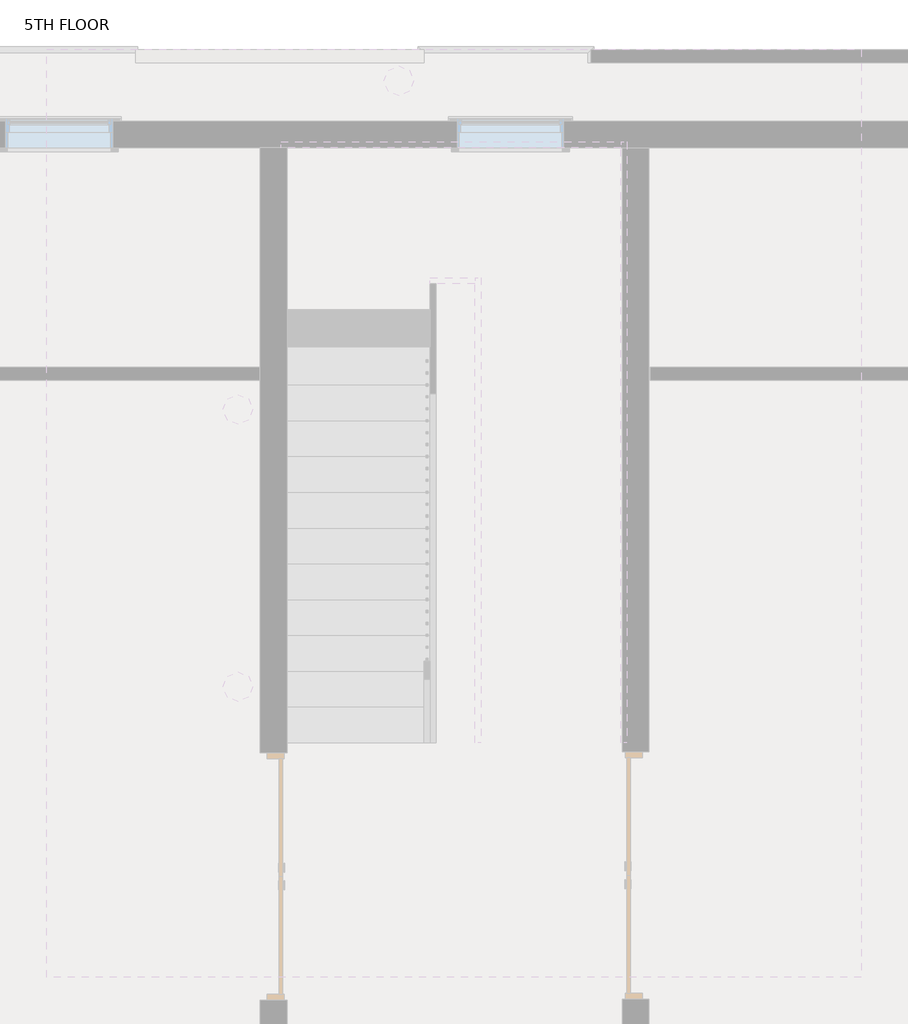
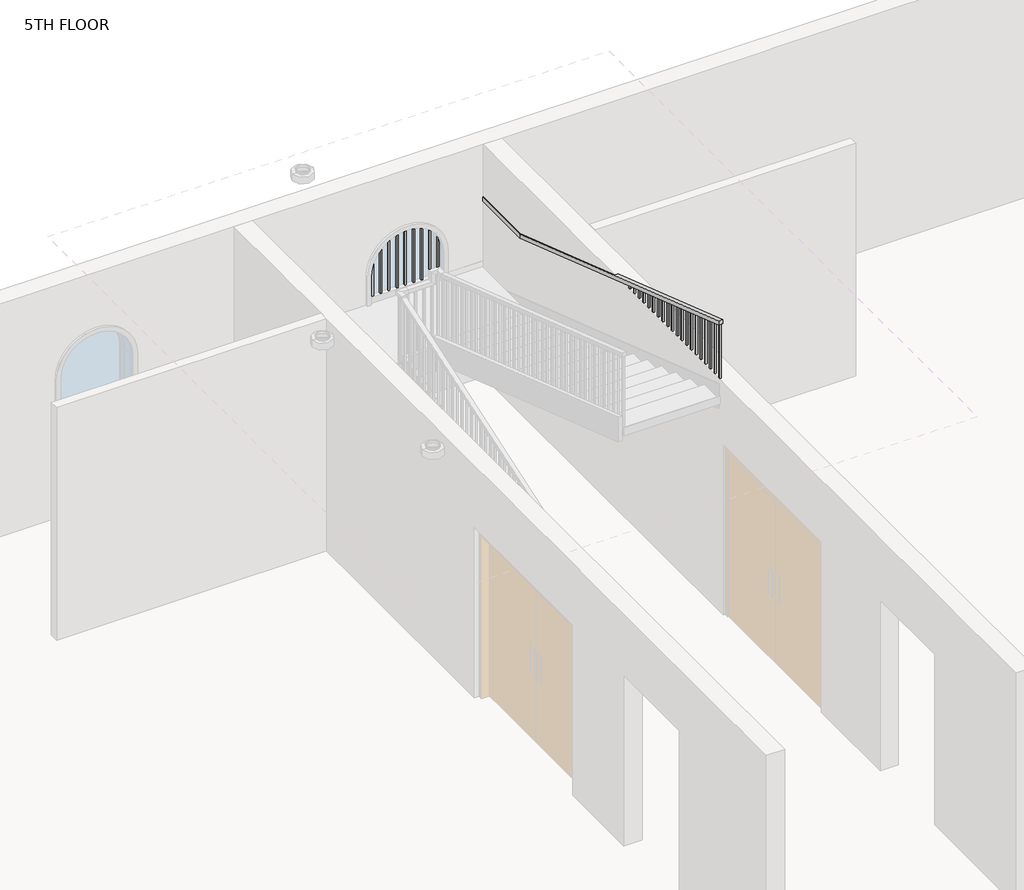
# One storey, part 5 of 7: 1 railing.
"""IFC4 building model written with IfcOpenShell, lengths in millimetres."""

from ifc_helpers import new_model, si_unit, frame, origin, place, context, project, spatial, polyline, outline, extrude, faceted_brep, element, save

model = new_model("IFC4")

# Units and contexts
model_context = context("Model", 3, world=origin())
ifc_project = project(units=[si_unit("LENGTHUNIT", "METRE", prefix="MILLI")], contexts=[model_context])

# Site, building, storey
site = spatial("IfcSite", under=ifc_project)
building = spatial("IfcBuilding", under=site)
storey = spatial("IfcBuildingStorey", under=building, Name="5TH FLOOR", Elevation=16002.0)

# Railing
placement = place(None, origin())
element("IfcRailing", 1, ObjectType="Handrail - Rectangular", at=placement, inside=storey, context=model_context, shape_type="SolidModel", body=[
    faceted_brep([(-1899.5987998, 2564.5067329, 17019.8142857), (-1899.5987998, 2564.5067329, 16966.1699957), (-1848.7987998, 2564.5067329, 16966.1699957), (-1848.7987998, 2564.5067329, 17019.8142857), (-1899.5987998, 6526.9067329, 18364.2), (-1899.5987998, 6535.2899033, 18313.4), (-1848.7987998, 6535.2899033, 18313.4), (-1848.7987998, 6526.9067329, 18364.2), (-1899.5987998, 7682.6067329, 18313.4), (-1899.5987998, 7682.6067329, 18364.2), (1046.8012002, 7682.6067329, 18364.2), (1046.8012002, 7682.6067329, 18313.4), (-1848.7987998, 7631.8067329, 18313.4), (996.0012002, 7631.8067329, 18313.4), (-1848.7987998, 7631.8067329, 18364.2), (996.0012002, 7631.8067329, 18364.2), (1046.8012002, 6831.7067329, 18364.2), (1046.8012002, 6823.3235624, 18313.4), (996.0012002, 6823.3235624, 18313.4), (996.0012002, 6831.7067329, 18364.2), (1046.8012002, 2564.5067329, 19812.0), (996.0012002, 2564.5067329, 19812.0), (996.0012002, 2564.5067329, 19758.35571), (1046.8012002, 2564.5067329, 19758.35571)], [[[0, 1, 2, 3]], [[1, 0, 4, 5]], [[2, 1, 5, 6]], [[3, 2, 6, 7]], [[0, 3, 7, 4]], [[8, 9, 10, 11]], [[12, 8, 11, 13]], [[14, 12, 13, 15]], [[9, 14, 15, 10]], [[11, 10, 16, 17]], [[13, 11, 17, 18]], [[15, 13, 18, 19]], [[10, 15, 19, 16]], [[5, 4, 9, 8]], [[6, 5, 8, 12]], [[7, 6, 12, 14]], [[4, 7, 14, 9]], [[20, 21, 22, 23]], [[17, 16, 20, 23]], [[18, 17, 23, 22]], [[19, 18, 22, 21]], [[16, 19, 21, 20]]]),
    extrude(outline(polyline([(2586.7317329, 19750.815085), (2586.7317329, 18979.8831452), (2567.6817329, 18986.3465381), (2567.6817329, 19757.2784779), (2586.7317329, 19750.815085)])), frame((1011.8762002, 0.0, 0.0), z_axis=(1.0, 0.0, 0.0), x_axis=(0.0, 1.0, 0.0)), (0.0, 0.0, 1.0), 19.05),
    extrude(outline(polyline([(2688.3317329, 19716.3436565), (2688.3317329, 18945.4117167), (2669.2817329, 18951.8751095), (2669.2817329, 19722.8070493), (2688.3317329, 19716.3436565)])), frame((1011.8762002, 0.0, 0.0), z_axis=(1.0, 0.0, 0.0), x_axis=(0.0, 1.0, 0.0)), (0.0, 0.0, 1.0), 19.05),
    extrude(outline(polyline([(2789.9317329, 19681.8722279), (2789.9317329, 18910.9402881), (2770.8817329, 18917.403681), (2770.8817329, 19688.3356207), (2789.9317329, 19681.8722279)])), frame((1011.8762002, 0.0, 0.0), z_axis=(1.0, 0.0, 0.0), x_axis=(0.0, 1.0, 0.0)), (0.0, 0.0, 1.0), 19.05),
    extrude(outline(polyline([(2891.5317329, 19647.4007993), (2891.5317329, 18876.4688595), (2872.4817329, 18882.9322524), (2872.4817329, 19653.8641922), (2891.5317329, 19647.4007993)])), frame((1011.8762002, 0.0, 0.0), z_axis=(1.0, 0.0, 0.0), x_axis=(0.0, 1.0, 0.0)), (0.0, 0.0, 1.0), 19.05),
    extrude(outline(polyline([(2993.1317329, 19612.9293707), (2993.1317329, 18841.997431), (2974.0817329, 18848.4608238), (2974.0817329, 19619.3927636), (2993.1317329, 19612.9293707)])), frame((1011.8762002, 0.0, 0.0), z_axis=(1.0, 0.0, 0.0), x_axis=(0.0, 1.0, 0.0)), (0.0, 0.0, 1.0), 19.05),
    extrude(outline(polyline([(3094.7317329, 19578.4579422), (3094.7317329, 18807.5260024), (3075.6817329, 18813.9893952), (3075.6817329, 19584.921335), (3094.7317329, 19578.4579422)])), frame((1011.8762002, 0.0, 0.0), z_axis=(1.0, 0.0, 0.0), x_axis=(0.0, 1.0, 0.0)), (0.0, 0.0, 1.0), 19.05),
    extrude(outline(polyline([(3196.3317329, 19543.9865136), (3196.3317329, 18773.0545738), (3177.2817329, 18779.5179667), (3177.2817329, 19550.4499065), (3196.3317329, 19543.9865136)])), frame((1011.8762002, 0.0, 0.0), z_axis=(1.0, 0.0, 0.0), x_axis=(0.0, 1.0, 0.0)), (0.0, 0.0, 1.0), 19.05),
    extrude(outline(polyline([(3297.9317329, 19509.515085), (3297.9317329, 18738.5831452), (3278.8817329, 18745.0465381), (3278.8817329, 19515.9784779), (3297.9317329, 19509.515085)])), frame((1011.8762002, 0.0, 0.0), z_axis=(1.0, 0.0, 0.0), x_axis=(0.0, 1.0, 0.0)), (0.0, 0.0, 1.0), 19.05),
    extrude(outline(polyline([(3399.5317329, 19475.0436565), (3399.5317329, 18704.1117167), (3380.4817329, 18710.5751095), (3380.4817329, 19481.5070493), (3399.5317329, 19475.0436565)])), frame((1011.8762002, 0.0, 0.0), z_axis=(1.0, 0.0, 0.0), x_axis=(0.0, 1.0, 0.0)), (0.0, 0.0, 1.0), 19.05),
    extrude(outline(polyline([(3501.1317329, 19440.5722279), (3501.1317329, 18669.6402881), (3482.0817329, 18676.103681), (3482.0817329, 19447.0356207), (3501.1317329, 19440.5722279)])), frame((1011.8762002, 0.0, 0.0), z_axis=(1.0, 0.0, 0.0), x_axis=(0.0, 1.0, 0.0)), (0.0, 0.0, 1.0), 19.05),
    extrude(outline(polyline([(3602.7317329, 19406.1007993), (3602.7317329, 18635.1688595), (3583.6817329, 18641.6322524), (3583.6817329, 19412.5641922), (3602.7317329, 19406.1007993)])), frame((1011.8762002, 0.0, 0.0), z_axis=(1.0, 0.0, 0.0), x_axis=(0.0, 1.0, 0.0)), (0.0, 0.0, 1.0), 19.05),
    extrude(outline(polyline([(3704.3317329, 19371.6293707), (3704.3317329, 18600.697431), (3685.2817329, 18607.1608238), (3685.2817329, 19378.0927636), (3704.3317329, 19371.6293707)])), frame((1011.8762002, 0.0, 0.0), z_axis=(1.0, 0.0, 0.0), x_axis=(0.0, 1.0, 0.0)), (0.0, 0.0, 1.0), 19.05),
    extrude(outline(polyline([(3805.9317329, 19337.1579422), (3805.9317329, 18566.2260024), (3786.8817329, 18572.6893952), (3786.8817329, 19343.621335), (3805.9317329, 19337.1579422)])), frame((1011.8762002, 0.0, 0.0), z_axis=(1.0, 0.0, 0.0), x_axis=(0.0, 1.0, 0.0)), (0.0, 0.0, 1.0), 19.05),
    extrude(outline(polyline([(3907.5317329, 19302.6865136), (3907.5317329, 18531.7545738), (3888.4817329, 18538.2179667), (3888.4817329, 19309.1499065), (3907.5317329, 19302.6865136)])), frame((1011.8762002, 0.0, 0.0), z_axis=(1.0, 0.0, 0.0), x_axis=(0.0, 1.0, 0.0)), (0.0, 0.0, 1.0), 19.05),
    extrude(outline(polyline([(4009.1317329, 19268.215085), (4009.1317329, 18497.2831452), (3990.0817329, 18503.7465381), (3990.0817329, 19274.6784779), (4009.1317329, 19268.215085)])), frame((1011.8762002, 0.0, 0.0), z_axis=(1.0, 0.0, 0.0), x_axis=(0.0, 1.0, 0.0)), (0.0, 0.0, 1.0), 19.05),
    extrude(outline(polyline([(4110.7317329, 19233.7436565), (4110.7317329, 18462.8117167), (4091.6817329, 18469.2751095), (4091.6817329, 19240.2070493), (4110.7317329, 19233.7436565)])), frame((1011.8762002, 0.0, 0.0), z_axis=(1.0, 0.0, 0.0), x_axis=(0.0, 1.0, 0.0)), (0.0, 0.0, 1.0), 19.05),
    extrude(outline(polyline([(4212.3317329, 19199.2722279), (4212.3317329, 18428.3402881), (4193.2817329, 18434.803681), (4193.2817329, 19205.7356207), (4212.3317329, 19199.2722279)])), frame((1011.8762002, 0.0, 0.0), z_axis=(1.0, 0.0, 0.0), x_axis=(0.0, 1.0, 0.0)), (0.0, 0.0, 1.0), 19.05),
    extrude(outline(polyline([(4313.9317329, 19164.8007993), (4313.9317329, 18393.8688595), (4294.8817329, 18400.3322524), (4294.8817329, 19171.2641922), (4313.9317329, 19164.8007993)])), frame((1011.8762002, 0.0, 0.0), z_axis=(1.0, 0.0, 0.0), x_axis=(0.0, 1.0, 0.0)), (0.0, 0.0, 1.0), 19.05),
    extrude(outline(polyline([(4415.5317329, 19130.3293707), (4415.5317329, 18359.397431), (4396.4817329, 18365.8608238), (4396.4817329, 19136.7927636), (4415.5317329, 19130.3293707)])), frame((1011.8762002, 0.0, 0.0), z_axis=(1.0, 0.0, 0.0), x_axis=(0.0, 1.0, 0.0)), (0.0, 0.0, 1.0), 19.05),
    extrude(outline(polyline([(4517.1317329, 19095.8579422), (4517.1317329, 18324.9260024), (4498.0817329, 18331.3893952), (4498.0817329, 19102.321335), (4517.1317329, 19095.8579422)])), frame((1011.8762002, 0.0, 0.0), z_axis=(1.0, 0.0, 0.0), x_axis=(0.0, 1.0, 0.0)), (0.0, 0.0, 1.0), 19.05),
    extrude(outline(polyline([(4618.7317329, 19061.3865136), (4618.7317329, 18290.4545738), (4599.6817329, 18296.9179667), (4599.6817329, 19067.8499065), (4618.7317329, 19061.3865136)])), frame((1011.8762002, 0.0, 0.0), z_axis=(1.0, 0.0, 0.0), x_axis=(0.0, 1.0, 0.0)), (0.0, 0.0, 1.0), 19.05),
    extrude(outline(polyline([(4720.3317329, 19026.915085), (4720.3317329, 18255.9831452), (4701.2817329, 18262.4465381), (4701.2817329, 19033.3784779), (4720.3317329, 19026.915085)])), frame((1011.8762002, 0.0, 0.0), z_axis=(1.0, 0.0, 0.0), x_axis=(0.0, 1.0, 0.0)), (0.0, 0.0, 1.0), 19.05),
    extrude(outline(polyline([(4821.9317329, 18992.4436565), (4821.9317329, 18221.5117167), (4802.8817329, 18227.9751095), (4802.8817329, 18998.9070493), (4821.9317329, 18992.4436565)])), frame((1011.8762002, 0.0, 0.0), z_axis=(1.0, 0.0, 0.0), x_axis=(0.0, 1.0, 0.0)), (0.0, 0.0, 1.0), 19.05),
    extrude(outline(polyline([(4923.5317329, 18957.9722279), (4923.5317329, 18187.0402881), (4904.4817329, 18193.503681), (4904.4817329, 18964.4356207), (4923.5317329, 18957.9722279)])), frame((1011.8762002, 0.0, 0.0), z_axis=(1.0, 0.0, 0.0), x_axis=(0.0, 1.0, 0.0)), (0.0, 0.0, 1.0), 19.05),
    extrude(outline(polyline([(5025.1317329, 18923.5007993), (5025.1317329, 18152.5688595), (5006.0817329, 18159.0322524), (5006.0817329, 18929.9641922), (5025.1317329, 18923.5007993)])), frame((1011.8762002, 0.0, 0.0), z_axis=(1.0, 0.0, 0.0), x_axis=(0.0, 1.0, 0.0)), (0.0, 0.0, 1.0), 19.05),
    extrude(outline(polyline([(5126.7317329, 18889.0293707), (5126.7317329, 18118.097431), (5107.6817329, 18124.5608238), (5107.6817329, 18895.4927636), (5126.7317329, 18889.0293707)])), frame((1011.8762002, 0.0, 0.0), z_axis=(1.0, 0.0, 0.0), x_axis=(0.0, 1.0, 0.0)), (0.0, 0.0, 1.0), 19.05),
    extrude(outline(polyline([(5228.3317329, 18854.5579422), (5228.3317329, 18083.6260024), (5209.2817329, 18090.0893952), (5209.2817329, 18861.021335), (5228.3317329, 18854.5579422)])), frame((1011.8762002, 0.0, 0.0), z_axis=(1.0, 0.0, 0.0), x_axis=(0.0, 1.0, 0.0)), (0.0, 0.0, 1.0), 19.05),
    extrude(outline(polyline([(5329.9317329, 18820.0865136), (5329.9317329, 18049.1545738), (5310.8817329, 18055.6179667), (5310.8817329, 18826.5499065), (5329.9317329, 18820.0865136)])), frame((1011.8762002, 0.0, 0.0), z_axis=(1.0, 0.0, 0.0), x_axis=(0.0, 1.0, 0.0)), (0.0, 0.0, 1.0), 19.05),
    extrude(outline(polyline([(5431.5317329, 18785.615085), (5431.5317329, 18014.6831452), (5412.4817329, 18021.1465381), (5412.4817329, 18792.0784779), (5431.5317329, 18785.615085)])), frame((1011.8762002, 0.0, 0.0), z_axis=(1.0, 0.0, 0.0), x_axis=(0.0, 1.0, 0.0)), (0.0, 0.0, 1.0), 19.05),
    extrude(outline(polyline([(5533.1317329, 18751.1436565), (5533.1317329, 17980.2117167), (5514.0817329, 17986.6751095), (5514.0817329, 18757.6070493), (5533.1317329, 18751.1436565)])), frame((1011.8762002, 0.0, 0.0), z_axis=(1.0, 0.0, 0.0), x_axis=(0.0, 1.0, 0.0)), (0.0, 0.0, 1.0), 19.05),
    extrude(outline(polyline([(5634.7317329, 18716.6722279), (5634.7317329, 17945.7402881), (5615.6817329, 17952.203681), (5615.6817329, 18723.1356207), (5634.7317329, 18716.6722279)])), frame((1011.8762002, 0.0, 0.0), z_axis=(1.0, 0.0, 0.0), x_axis=(0.0, 1.0, 0.0)), (0.0, 0.0, 1.0), 19.05),
    extrude(outline(polyline([(5736.3317329, 18682.2007993), (5736.3317329, 17911.2688595), (5717.2817329, 17917.7322524), (5717.2817329, 18688.6641922), (5736.3317329, 18682.2007993)])), frame((1011.8762002, 0.0, 0.0), z_axis=(1.0, 0.0, 0.0), x_axis=(0.0, 1.0, 0.0)), (0.0, 0.0, 1.0), 19.05),
    extrude(outline(polyline([(5837.9317329, 18647.7293707), (5837.9317329, 17876.797431), (5818.8817329, 17883.2608238), (5818.8817329, 18654.1927636), (5837.9317329, 18647.7293707)])), frame((1011.8762002, 0.0, 0.0), z_axis=(1.0, 0.0, 0.0), x_axis=(0.0, 1.0, 0.0)), (0.0, 0.0, 1.0), 19.05),
    extrude(outline(polyline([(5939.5317329, 18613.2579422), (5939.5317329, 17842.3260024), (5920.4817329, 17848.7893952), (5920.4817329, 18619.721335), (5939.5317329, 18613.2579422)])), frame((1011.8762002, 0.0, 0.0), z_axis=(1.0, 0.0, 0.0), x_axis=(0.0, 1.0, 0.0)), (0.0, 0.0, 1.0), 19.05),
    extrude(outline(polyline([(6041.1317329, 18578.7865136), (6041.1317329, 17807.8545738), (6022.0817329, 17814.3179667), (6022.0817329, 18585.2499065), (6041.1317329, 18578.7865136)])), frame((1011.8762002, 0.0, 0.0), z_axis=(1.0, 0.0, 0.0), x_axis=(0.0, 1.0, 0.0)), (0.0, 0.0, 1.0), 19.05),
    extrude(outline(polyline([(6142.7317329, 18544.315085), (6142.7317329, 17773.3831452), (6123.6817329, 17779.8465381), (6123.6817329, 18550.7784779), (6142.7317329, 18544.315085)])), frame((1011.8762002, 0.0, 0.0), z_axis=(1.0, 0.0, 0.0), x_axis=(0.0, 1.0, 0.0)), (0.0, 0.0, 1.0), 19.05),
    extrude(outline(polyline([(6244.3317329, 18509.8436565), (6244.3317329, 17738.9117167), (6225.2817329, 17745.3751095), (6225.2817329, 18516.3070493), (6244.3317329, 18509.8436565)])), frame((1011.8762002, 0.0, 0.0), z_axis=(1.0, 0.0, 0.0), x_axis=(0.0, 1.0, 0.0)), (0.0, 0.0, 1.0), 19.05),
    extrude(outline(polyline([(6345.9317329, 18475.3722279), (6345.9317329, 17704.4402881), (6326.8817329, 17710.903681), (6326.8817329, 18481.8356207), (6345.9317329, 18475.3722279)])), frame((1011.8762002, 0.0, 0.0), z_axis=(1.0, 0.0, 0.0), x_axis=(0.0, 1.0, 0.0)), (0.0, 0.0, 1.0), 19.05),
    extrude(outline(polyline([(6447.5317329, 18440.9007993), (6447.5317329, 17669.9688595), (6428.4817329, 17676.4322524), (6428.4817329, 18447.3641922), (6447.5317329, 18440.9007993)])), frame((1011.8762002, 0.0, 0.0), z_axis=(1.0, 0.0, 0.0), x_axis=(0.0, 1.0, 0.0)), (0.0, 0.0, 1.0), 19.05),
    extrude(outline(polyline([(6549.1317329, 18406.4293707), (6549.1317329, 17635.497431), (6530.0817329, 17641.9608238), (6530.0817329, 18412.8927636), (6549.1317329, 18406.4293707)])), frame((1011.8762002, 0.0, 0.0), z_axis=(1.0, 0.0, 0.0), x_axis=(0.0, 1.0, 0.0)), (0.0, 0.0, 1.0), 19.05),
    extrude(outline(polyline([(6650.7317329, 18371.9579422), (6650.7317329, 17601.0260024), (6631.6817329, 17607.4893952), (6631.6817329, 18378.421335), (6650.7317329, 18371.9579422)])), frame((1011.8762002, 0.0, 0.0), z_axis=(1.0, 0.0, 0.0), x_axis=(0.0, 1.0, 0.0)), (0.0, 0.0, 1.0), 19.05),
    extrude(outline(polyline([(6752.3317329, 18337.4865136), (6752.3317329, 17566.5545738), (6733.2817329, 17573.0179667), (6733.2817329, 18343.9499065), (6752.3317329, 18337.4865136)])), frame((1011.8762002, 0.0, 0.0), z_axis=(1.0, 0.0, 0.0), x_axis=(0.0, 1.0, 0.0)), (0.0, 0.0, 1.0), 19.05),
    extrude(outline(polyline([(6853.9317329, 18313.4), (6853.9317329, 17532.0831452), (6834.8817329, 17538.5465381), (6834.8817329, 18313.4), (6853.9317329, 18313.4)])), frame((1011.8762002, 0.0, 0.0), z_axis=(1.0, 0.0, 0.0), x_axis=(0.0, 1.0, 0.0)), (0.0, 0.0, 1.0), 19.05),
    extrude(outline(polyline([(6955.5317329, 18313.4), (6955.5317329, 17497.6117167), (6936.4817329, 17504.0751095), (6936.4817329, 18313.4), (6955.5317329, 18313.4)])), frame((1011.8762002, 0.0, 0.0), z_axis=(1.0, 0.0, 0.0), x_axis=(0.0, 1.0, 0.0)), (0.0, 0.0, 1.0), 19.05),
    extrude(outline(polyline([(7057.1317329, 18313.4), (7057.1317329, 17463.1402881), (7038.0817329, 17469.603681), (7038.0817329, 18313.4), (7057.1317329, 18313.4)])), frame((1011.8762002, 0.0, 0.0), z_axis=(1.0, 0.0, 0.0), x_axis=(0.0, 1.0, 0.0)), (0.0, 0.0, 1.0), 19.05),
    extrude(outline(polyline([(7158.7317329, 18313.4), (7158.7317329, 17428.6688595), (7139.6817329, 17435.1322524), (7139.6817329, 18313.4), (7158.7317329, 18313.4)])), frame((1011.8762002, 0.0, 0.0), z_axis=(1.0, 0.0, 0.0), x_axis=(0.0, 1.0, 0.0)), (0.0, 0.0, 1.0), 19.05),
    extrude(outline(polyline([(7260.3317329, 18313.4), (7260.3317329, 17394.197431), (7241.2817329, 17400.6608238), (7241.2817329, 18313.4), (7260.3317329, 18313.4)])), frame((1011.8762002, 0.0, 0.0), z_axis=(1.0, 0.0, 0.0), x_axis=(0.0, 1.0, 0.0)), (0.0, 0.0, 1.0), 19.05),
    extrude(outline(polyline([(7361.9317329, 18313.4), (7361.9317329, 17359.7260024), (7342.8817329, 17366.1893952), (7342.8817329, 18313.4), (7361.9317329, 18313.4)])), frame((1011.8762002, 0.0, 0.0), z_axis=(1.0, 0.0, 0.0), x_axis=(0.0, 1.0, 0.0)), (0.0, 0.0, 1.0), 19.05),
    extrude(outline(polyline([(7463.5317329, 18313.4), (7463.5317329, 17325.2545738), (7444.4817329, 17331.7179667), (7444.4817329, 18313.4), (7463.5317329, 18313.4)])), frame((1011.8762002, 0.0, 0.0), z_axis=(1.0, 0.0, 0.0), x_axis=(0.0, 1.0, 0.0)), (0.0, 0.0, 1.0), 19.05),
    extrude(outline(polyline([(7565.1317329, 18313.4), (7565.1317329, 17290.7831452), (7546.0817329, 17297.2465381), (7546.0817329, 18313.4), (7565.1317329, 18313.4)])), frame((1011.8762002, 0.0, 0.0), z_axis=(1.0, 0.0, 0.0), x_axis=(0.0, 1.0, 0.0)), (0.0, 0.0, 1.0), 19.05),
    extrude(outline(polyline([(961.0762002, 7666.7317329), (980.1262002, 7666.7317329), (980.1262002, 7647.6817329), (961.0762002, 7647.6817329), (961.0762002, 7666.7317329)])), frame((0.0, 0.0, 17526.0), z_axis=(0.0, 0.0, 1.0), x_axis=(1.0, 0.0, 0.0)), (0.0, 0.0, 1.0), 787.4),
    extrude(outline(polyline([(859.4762002, 7666.7317329), (878.5262002, 7666.7317329), (878.5262002, 7647.6817329), (859.4762002, 7647.6817329), (859.4762002, 7666.7317329)])), frame((0.0, 0.0, 17526.0), z_axis=(0.0, 0.0, 1.0), x_axis=(1.0, 0.0, 0.0)), (0.0, 0.0, 1.0), 787.4),
    extrude(outline(polyline([(757.8762002, 7666.7317329), (776.9262002, 7666.7317329), (776.9262002, 7647.6817329), (757.8762002, 7647.6817329), (757.8762002, 7666.7317329)])), frame((0.0, 0.0, 17526.0), z_axis=(0.0, 0.0, 1.0), x_axis=(1.0, 0.0, 0.0)), (0.0, 0.0, 1.0), 787.4),
    extrude(outline(polyline([(656.2762002, 7666.7317329), (675.3262002, 7666.7317329), (675.3262002, 7647.6817329), (656.2762002, 7647.6817329), (656.2762002, 7666.7317329)])), frame((0.0, 0.0, 17526.0), z_axis=(0.0, 0.0, 1.0), x_axis=(1.0, 0.0, 0.0)), (0.0, 0.0, 1.0), 787.4),
    extrude(outline(polyline([(554.6762002, 7666.7317329), (573.7262002, 7666.7317329), (573.7262002, 7647.6817329), (554.6762002, 7647.6817329), (554.6762002, 7666.7317329)])), frame((0.0, 0.0, 17526.0), z_axis=(0.0, 0.0, 1.0), x_axis=(1.0, 0.0, 0.0)), (0.0, 0.0, 1.0), 787.4),
    extrude(outline(polyline([(453.0762002, 7666.7317329), (472.1262002, 7666.7317329), (472.1262002, 7647.6817329), (453.0762002, 7647.6817329), (453.0762002, 7666.7317329)])), frame((0.0, 0.0, 17526.0), z_axis=(0.0, 0.0, 1.0), x_axis=(1.0, 0.0, 0.0)), (0.0, 0.0, 1.0), 787.4),
    extrude(outline(polyline([(351.4762002, 7666.7317329), (370.5262002, 7666.7317329), (370.5262002, 7647.6817329), (351.4762002, 7647.6817329), (351.4762002, 7666.7317329)])), frame((0.0, 0.0, 17526.0), z_axis=(0.0, 0.0, 1.0), x_axis=(1.0, 0.0, 0.0)), (0.0, 0.0, 1.0), 787.4),
    extrude(outline(polyline([(249.8762002, 7666.7317329), (268.9262002, 7666.7317329), (268.9262002, 7647.6817329), (249.8762002, 7647.6817329), (249.8762002, 7666.7317329)])), frame((0.0, 0.0, 17526.0), z_axis=(0.0, 0.0, 1.0), x_axis=(1.0, 0.0, 0.0)), (0.0, 0.0, 1.0), 787.4),
    extrude(outline(polyline([(148.2762002, 7666.7317329), (167.3262002, 7666.7317329), (167.3262002, 7647.6817329), (148.2762002, 7647.6817329), (148.2762002, 7666.7317329)])), frame((0.0, 0.0, 17526.0), z_axis=(0.0, 0.0, 1.0), x_axis=(1.0, 0.0, 0.0)), (0.0, 0.0, 1.0), 787.4),
    extrude(outline(polyline([(46.6762002, 7666.7317329), (65.7262002, 7666.7317329), (65.7262002, 7647.6817329), (46.6762002, 7647.6817329), (46.6762002, 7666.7317329)])), frame((0.0, 0.0, 17526.0), z_axis=(0.0, 0.0, 1.0), x_axis=(1.0, 0.0, 0.0)), (0.0, 0.0, 1.0), 787.4),
    extrude(outline(polyline([(-54.9237998, 7666.7317329), (-35.8737998, 7666.7317329), (-35.8737998, 7647.6817329), (-54.9237998, 7647.6817329), (-54.9237998, 7666.7317329)])), frame((0.0, 0.0, 17526.0), z_axis=(0.0, 0.0, 1.0), x_axis=(1.0, 0.0, 0.0)), (0.0, 0.0, 1.0), 787.4),
    extrude(outline(polyline([(-156.5237998, 7666.7317329), (-137.4737998, 7666.7317329), (-137.4737998, 7647.6817329), (-156.5237998, 7647.6817329), (-156.5237998, 7666.7317329)])), frame((0.0, 0.0, 17526.0), z_axis=(0.0, 0.0, 1.0), x_axis=(1.0, 0.0, 0.0)), (0.0, 0.0, 1.0), 787.4),
    extrude(outline(polyline([(-258.1237998, 7666.7317329), (-239.0737998, 7666.7317329), (-239.0737998, 7647.6817329), (-258.1237998, 7647.6817329), (-258.1237998, 7666.7317329)])), frame((0.0, 0.0, 17526.0), z_axis=(0.0, 0.0, 1.0), x_axis=(1.0, 0.0, 0.0)), (0.0, 0.0, 1.0), 787.4),
    extrude(outline(polyline([(-359.7237998, 7666.7317329), (-340.6737998, 7666.7317329), (-340.6737998, 7647.6817329), (-359.7237998, 7647.6817329), (-359.7237998, 7666.7317329)])), frame((0.0, 0.0, 17526.0), z_axis=(0.0, 0.0, 1.0), x_axis=(1.0, 0.0, 0.0)), (0.0, 0.0, 1.0), 787.4),
    extrude(outline(polyline([(-461.3237998, 7666.7317329), (-442.2737998, 7666.7317329), (-442.2737998, 7647.6817329), (-461.3237998, 7647.6817329), (-461.3237998, 7666.7317329)])), frame((0.0, 0.0, 17526.0), z_axis=(0.0, 0.0, 1.0), x_axis=(1.0, 0.0, 0.0)), (0.0, 0.0, 1.0), 787.4),
    extrude(outline(polyline([(-562.9237998, 7666.7317329), (-543.8737998, 7666.7317329), (-543.8737998, 7647.6817329), (-562.9237998, 7647.6817329), (-562.9237998, 7666.7317329)])), frame((0.0, 0.0, 17526.0), z_axis=(0.0, 0.0, 1.0), x_axis=(1.0, 0.0, 0.0)), (0.0, 0.0, 1.0), 787.4),
    extrude(outline(polyline([(-664.5237998, 7666.7317329), (-645.4737998, 7666.7317329), (-645.4737998, 7647.6817329), (-664.5237998, 7647.6817329), (-664.5237998, 7666.7317329)])), frame((0.0, 0.0, 17526.0), z_axis=(0.0, 0.0, 1.0), x_axis=(1.0, 0.0, 0.0)), (0.0, 0.0, 1.0), 787.4),
    extrude(outline(polyline([(-766.1237998, 7666.7317329), (-747.0737998, 7666.7317329), (-747.0737998, 7647.6817329), (-766.1237998, 7647.6817329), (-766.1237998, 7666.7317329)])), frame((0.0, 0.0, 17526.0), z_axis=(0.0, 0.0, 1.0), x_axis=(1.0, 0.0, 0.0)), (0.0, 0.0, 1.0), 787.4),
    extrude(outline(polyline([(-867.7237998, 7666.7317329), (-848.6737998, 7666.7317329), (-848.6737998, 7647.6817329), (-867.7237998, 7647.6817329), (-867.7237998, 7666.7317329)])), frame((0.0, 0.0, 17526.0), z_axis=(0.0, 0.0, 1.0), x_axis=(1.0, 0.0, 0.0)), (0.0, 0.0, 1.0), 787.4),
    extrude(outline(polyline([(-969.3237998, 7666.7317329), (-950.2737998, 7666.7317329), (-950.2737998, 7647.6817329), (-969.3237998, 7647.6817329), (-969.3237998, 7666.7317329)])), frame((0.0, 0.0, 17526.0), z_axis=(0.0, 0.0, 1.0), x_axis=(1.0, 0.0, 0.0)), (0.0, 0.0, 1.0), 787.4),
    extrude(outline(polyline([(-1070.9237998, 7666.7317329), (-1051.8737998, 7666.7317329), (-1051.8737998, 7647.6817329), (-1070.9237998, 7647.6817329), (-1070.9237998, 7666.7317329)])), frame((0.0, 0.0, 17526.0), z_axis=(0.0, 0.0, 1.0), x_axis=(1.0, 0.0, 0.0)), (0.0, 0.0, 1.0), 787.4),
    extrude(outline(polyline([(-1172.5237998, 7666.7317329), (-1153.4737998, 7666.7317329), (-1153.4737998, 7647.6817329), (-1172.5237998, 7647.6817329), (-1172.5237998, 7666.7317329)])), frame((0.0, 0.0, 17526.0), z_axis=(0.0, 0.0, 1.0), x_axis=(1.0, 0.0, 0.0)), (0.0, 0.0, 1.0), 787.4),
    extrude(outline(polyline([(-1274.1237998, 7666.7317329), (-1255.0737998, 7666.7317329), (-1255.0737998, 7647.6817329), (-1274.1237998, 7647.6817329), (-1274.1237998, 7666.7317329)])), frame((0.0, 0.0, 17526.0), z_axis=(0.0, 0.0, 1.0), x_axis=(1.0, 0.0, 0.0)), (0.0, 0.0, 1.0), 787.4),
    extrude(outline(polyline([(-1375.7237998, 7666.7317329), (-1356.6737998, 7666.7317329), (-1356.6737998, 7647.6817329), (-1375.7237998, 7647.6817329), (-1375.7237998, 7666.7317329)])), frame((0.0, 0.0, 17526.0), z_axis=(0.0, 0.0, 1.0), x_axis=(1.0, 0.0, 0.0)), (0.0, 0.0, 1.0), 787.4),
    extrude(outline(polyline([(-1477.3237998, 7666.7317329), (-1458.2737998, 7666.7317329), (-1458.2737998, 7647.6817329), (-1477.3237998, 7647.6817329), (-1477.3237998, 7666.7317329)])), frame((0.0, 0.0, 17526.0), z_axis=(0.0, 0.0, 1.0), x_axis=(1.0, 0.0, 0.0)), (0.0, 0.0, 1.0), 787.4),
    extrude(outline(polyline([(-1578.9237998, 7666.7317329), (-1559.8737998, 7666.7317329), (-1559.8737998, 7647.6817329), (-1578.9237998, 7647.6817329), (-1578.9237998, 7666.7317329)])), frame((0.0, 0.0, 17526.0), z_axis=(0.0, 0.0, 1.0), x_axis=(1.0, 0.0, 0.0)), (0.0, 0.0, 1.0), 787.4),
    extrude(outline(polyline([(-1680.5237998, 7666.7317329), (-1661.4737998, 7666.7317329), (-1661.4737998, 7647.6817329), (-1680.5237998, 7647.6817329), (-1680.5237998, 7666.7317329)])), frame((0.0, 0.0, 17526.0), z_axis=(0.0, 0.0, 1.0), x_axis=(1.0, 0.0, 0.0)), (0.0, 0.0, 1.0), 787.4),
    extrude(outline(polyline([(-1782.1237998, 7666.7317329), (-1763.0737998, 7666.7317329), (-1763.0737998, 7647.6817329), (-1782.1237998, 7647.6817329), (-1782.1237998, 7666.7317329)])), frame((0.0, 0.0, 17526.0), z_axis=(0.0, 0.0, 1.0), x_axis=(1.0, 0.0, 0.0)), (0.0, 0.0, 1.0), 787.4),
    extrude(outline(polyline([(-1883.7237998, 7634.9817329), (-1883.7237998, 7654.0317329), (-1864.6737998, 7654.0317329), (-1864.6737998, 7634.9817329), (-1883.7237998, 7634.9817329)])), frame((0.0, 0.0, 17828.9857143), z_axis=(0.0, 0.0, 1.0), x_axis=(1.0, 0.0, 0.0)), (0.0, 0.0, 1.0), 484.4142857),
    extrude(outline(polyline([(-1883.7237998, 7533.3817329), (-1883.7237998, 7552.4317329), (-1864.6737998, 7552.4317329), (-1864.6737998, 7533.3817329), (-1883.7237998, 7533.3817329)])), frame((0.0, 0.0, 17794.5142857), z_axis=(0.0, 0.0, 1.0), x_axis=(1.0, 0.0, 0.0)), (0.0, 0.0, 1.0), 518.8857143),
    extrude(outline(polyline([(-1883.7237998, 7431.7817329), (-1883.7237998, 7450.8317329), (-1864.6737998, 7450.8317329), (-1864.6737998, 7431.7817329), (-1883.7237998, 7431.7817329)])), frame((0.0, 0.0, 17760.0428571), z_axis=(0.0, 0.0, 1.0), x_axis=(1.0, 0.0, 0.0)), (0.0, 0.0, 1.0), 553.3571429),
    extrude(outline(polyline([(-1883.7237998, 7330.1817329), (-1883.7237998, 7349.2317329), (-1864.6737998, 7349.2317329), (-1864.6737998, 7330.1817329), (-1883.7237998, 7330.1817329)])), frame((0.0, 0.0, 17725.5714286), z_axis=(0.0, 0.0, 1.0), x_axis=(1.0, 0.0, 0.0)), (0.0, 0.0, 1.0), 587.8285714),
    extrude(outline(polyline([(-1883.7237998, 7228.5817329), (-1883.7237998, 7247.6317329), (-1864.6737998, 7247.6317329), (-1864.6737998, 7228.5817329), (-1883.7237998, 7228.5817329)])), frame((0.0, 0.0, 17691.1), z_axis=(0.0, 0.0, 1.0), x_axis=(1.0, 0.0, 0.0)), (0.0, 0.0, 1.0), 622.3),
    extrude(outline(polyline([(-1883.7237998, 7126.9817329), (-1883.7237998, 7146.0317329), (-1864.6737998, 7146.0317329), (-1864.6737998, 7126.9817329), (-1883.7237998, 7126.9817329)])), frame((0.0, 0.0, 17656.6285714), z_axis=(0.0, 0.0, 1.0), x_axis=(1.0, 0.0, 0.0)), (0.0, 0.0, 1.0), 656.7714286),
    extrude(outline(polyline([(-1883.7237998, 7025.3817329), (-1883.7237998, 7044.4317329), (-1864.6737998, 7044.4317329), (-1864.6737998, 7025.3817329), (-1883.7237998, 7025.3817329)])), frame((0.0, 0.0, 17526.0), z_axis=(0.0, 0.0, 1.0), x_axis=(1.0, 0.0, 0.0)), (0.0, 0.0, 1.0), 787.4),
    extrude(outline(polyline([(-1883.7237998, 6923.7817329), (-1883.7237998, 6942.8317329), (-1864.6737998, 6942.8317329), (-1864.6737998, 6923.7817329), (-1883.7237998, 6923.7817329)])), frame((0.0, 0.0, 17526.0), z_axis=(0.0, 0.0, 1.0), x_axis=(1.0, 0.0, 0.0)), (0.0, 0.0, 1.0), 787.4),
    extrude(outline(polyline([(-1883.7237998, 6822.1817329), (-1883.7237998, 6841.2317329), (-1864.6737998, 6841.2317329), (-1864.6737998, 6822.1817329), (-1883.7237998, 6822.1817329)])), frame((0.0, 0.0, 17526.0), z_axis=(0.0, 0.0, 1.0), x_axis=(1.0, 0.0, 0.0)), (0.0, 0.0, 1.0), 787.4),
    extrude(outline(polyline([(-1883.7237998, 6720.5817329), (-1883.7237998, 6739.6317329), (-1864.6737998, 6739.6317329), (-1864.6737998, 6720.5817329), (-1883.7237998, 6720.5817329)])), frame((0.0, 0.0, 17526.0), z_axis=(0.0, 0.0, 1.0), x_axis=(1.0, 0.0, 0.0)), (0.0, 0.0, 1.0), 787.4),
    extrude(outline(polyline([(-1883.7237998, 6618.9817329), (-1883.7237998, 6638.0317329), (-1864.6737998, 6638.0317329), (-1864.6737998, 6618.9817329), (-1883.7237998, 6618.9817329)])), frame((0.0, 0.0, 17526.0), z_axis=(0.0, 0.0, 1.0), x_axis=(1.0, 0.0, 0.0)), (0.0, 0.0, 1.0), 787.4),
    extrude(outline(polyline([(6536.4317329, 18313.7874065), (6536.4317329, 17526.0), (6517.3817329, 17526.0), (6517.3817329, 18307.3240136), (6536.4317329, 18313.7874065)])), frame((-1883.7237998, 0.0, 0.0), z_axis=(1.0, 0.0, 0.0), x_axis=(0.0, 1.0, 0.0)), (0.0, 0.0, 1.0), 19.05),
    extrude(outline(polyline([(6434.8317329, 18279.3159779), (6434.8317329, 17508.3840381), (6415.7817329, 17501.9206452), (6415.7817329, 18272.852585), (6434.8317329, 18279.3159779)])), frame((-1883.7237998, 0.0, 0.0), z_axis=(1.0, 0.0, 0.0), x_axis=(0.0, 1.0, 0.0)), (0.0, 0.0, 1.0), 19.05),
    extrude(outline(polyline([(6333.2317329, 18244.8445493), (6333.2317329, 17473.9126095), (6314.1817329, 17467.4492167), (6314.1817329, 18238.3811565), (6333.2317329, 18244.8445493)])), frame((-1883.7237998, 0.0, 0.0), z_axis=(1.0, 0.0, 0.0), x_axis=(0.0, 1.0, 0.0)), (0.0, 0.0, 1.0), 19.05),
    extrude(outline(polyline([(6231.6317329, 18210.3731207), (6231.6317329, 17439.441181), (6212.5817329, 17432.9777881), (6212.5817329, 18203.9097279), (6231.6317329, 18210.3731207)])), frame((-1883.7237998, 0.0, 0.0), z_axis=(1.0, 0.0, 0.0), x_axis=(0.0, 1.0, 0.0)), (0.0, 0.0, 1.0), 19.05),
    extrude(outline(polyline([(6130.0317329, 18175.9016922), (6130.0317329, 17404.9697524), (6110.9817329, 17398.5063595), (6110.9817329, 18169.4382993), (6130.0317329, 18175.9016922)])), frame((-1883.7237998, 0.0, 0.0), z_axis=(1.0, 0.0, 0.0), x_axis=(0.0, 1.0, 0.0)), (0.0, 0.0, 1.0), 19.05),
    extrude(outline(polyline([(6028.4317329, 18141.4302636), (6028.4317329, 17370.4983238), (6009.3817329, 17364.034931), (6009.3817329, 18134.9668707), (6028.4317329, 18141.4302636)])), frame((-1883.7237998, 0.0, 0.0), z_axis=(1.0, 0.0, 0.0), x_axis=(0.0, 1.0, 0.0)), (0.0, 0.0, 1.0), 19.05),
    extrude(outline(polyline([(5926.8317329, 18106.958835), (5926.8317329, 17336.0268952), (5907.7817329, 17329.5635024), (5907.7817329, 18100.4954422), (5926.8317329, 18106.958835)])), frame((-1883.7237998, 0.0, 0.0), z_axis=(1.0, 0.0, 0.0), x_axis=(0.0, 1.0, 0.0)), (0.0, 0.0, 1.0), 19.05),
    extrude(outline(polyline([(5825.2317329, 18072.4874065), (5825.2317329, 17301.5554667), (5806.1817329, 17295.0920738), (5806.1817329, 18066.0240136), (5825.2317329, 18072.4874065)])), frame((-1883.7237998, 0.0, 0.0), z_axis=(1.0, 0.0, 0.0), x_axis=(0.0, 1.0, 0.0)), (0.0, 0.0, 1.0), 19.05),
    extrude(outline(polyline([(5723.6317329, 18038.0159779), (5723.6317329, 17267.0840381), (5704.5817329, 17260.6206452), (5704.5817329, 18031.552585), (5723.6317329, 18038.0159779)])), frame((-1883.7237998, 0.0, 0.0), z_axis=(1.0, 0.0, 0.0), x_axis=(0.0, 1.0, 0.0)), (0.0, 0.0, 1.0), 19.05),
    extrude(outline(polyline([(5622.0317329, 18003.5445493), (5622.0317329, 17232.6126095), (5602.9817329, 17226.1492167), (5602.9817329, 17997.0811565), (5622.0317329, 18003.5445493)])), frame((-1883.7237998, 0.0, 0.0), z_axis=(1.0, 0.0, 0.0), x_axis=(0.0, 1.0, 0.0)), (0.0, 0.0, 1.0), 19.05),
    extrude(outline(polyline([(5520.4317329, 17969.0731207), (5520.4317329, 17198.141181), (5501.3817329, 17191.6777881), (5501.3817329, 17962.6097279), (5520.4317329, 17969.0731207)])), frame((-1883.7237998, 0.0, 0.0), z_axis=(1.0, 0.0, 0.0), x_axis=(0.0, 1.0, 0.0)), (0.0, 0.0, 1.0), 19.05),
    extrude(outline(polyline([(5418.8317329, 17934.6016922), (5418.8317329, 17163.6697524), (5399.7817329, 17157.2063595), (5399.7817329, 17928.1382993), (5418.8317329, 17934.6016922)])), frame((-1883.7237998, 0.0, 0.0), z_axis=(1.0, 0.0, 0.0), x_axis=(0.0, 1.0, 0.0)), (0.0, 0.0, 1.0), 19.05),
    extrude(outline(polyline([(5317.2317329, 17900.1302636), (5317.2317329, 17129.1983238), (5298.1817329, 17122.734931), (5298.1817329, 17893.6668707), (5317.2317329, 17900.1302636)])), frame((-1883.7237998, 0.0, 0.0), z_axis=(1.0, 0.0, 0.0), x_axis=(0.0, 1.0, 0.0)), (0.0, 0.0, 1.0), 19.05),
    extrude(outline(polyline([(5215.6317329, 17865.658835), (5215.6317329, 17094.7268952), (5196.5817329, 17088.2635024), (5196.5817329, 17859.1954422), (5215.6317329, 17865.658835)])), frame((-1883.7237998, 0.0, 0.0), z_axis=(1.0, 0.0, 0.0), x_axis=(0.0, 1.0, 0.0)), (0.0, 0.0, 1.0), 19.05),
    extrude(outline(polyline([(5114.0317329, 17831.1874065), (5114.0317329, 17060.2554667), (5094.9817329, 17053.7920738), (5094.9817329, 17824.7240136), (5114.0317329, 17831.1874065)])), frame((-1883.7237998, 0.0, 0.0), z_axis=(1.0, 0.0, 0.0), x_axis=(0.0, 1.0, 0.0)), (0.0, 0.0, 1.0), 19.05),
    extrude(outline(polyline([(5012.4317329, 17796.7159779), (5012.4317329, 17025.7840381), (4993.3817329, 17019.3206452), (4993.3817329, 17790.252585), (5012.4317329, 17796.7159779)])), frame((-1883.7237998, 0.0, 0.0), z_axis=(1.0, 0.0, 0.0), x_axis=(0.0, 1.0, 0.0)), (0.0, 0.0, 1.0), 19.05),
    extrude(outline(polyline([(4910.8317329, 17762.2445493), (4910.8317329, 16991.3126095), (4891.7817329, 16984.8492167), (4891.7817329, 17755.7811565), (4910.8317329, 17762.2445493)])), frame((-1883.7237998, 0.0, 0.0), z_axis=(1.0, 0.0, 0.0), x_axis=(0.0, 1.0, 0.0)), (0.0, 0.0, 1.0), 19.05),
    extrude(outline(polyline([(4809.2317329, 17727.7731207), (4809.2317329, 16956.841181), (4790.1817329, 16950.3777881), (4790.1817329, 17721.3097279), (4809.2317329, 17727.7731207)])), frame((-1883.7237998, 0.0, 0.0), z_axis=(1.0, 0.0, 0.0), x_axis=(0.0, 1.0, 0.0)), (0.0, 0.0, 1.0), 19.05),
    extrude(outline(polyline([(4707.6317329, 17693.3016922), (4707.6317329, 16922.3697524), (4688.5817329, 16915.9063595), (4688.5817329, 17686.8382993), (4707.6317329, 17693.3016922)])), frame((-1883.7237998, 0.0, 0.0), z_axis=(1.0, 0.0, 0.0), x_axis=(0.0, 1.0, 0.0)), (0.0, 0.0, 1.0), 19.05),
    extrude(outline(polyline([(4606.0317329, 17658.8302636), (4606.0317329, 16887.8983238), (4586.9817329, 16881.434931), (4586.9817329, 17652.3668707), (4606.0317329, 17658.8302636)])), frame((-1883.7237998, 0.0, 0.0), z_axis=(1.0, 0.0, 0.0), x_axis=(0.0, 1.0, 0.0)), (0.0, 0.0, 1.0), 19.05),
    extrude(outline(polyline([(4504.4317329, 17624.358835), (4504.4317329, 16853.4268952), (4485.3817329, 16846.9635024), (4485.3817329, 17617.8954422), (4504.4317329, 17624.358835)])), frame((-1883.7237998, 0.0, 0.0), z_axis=(1.0, 0.0, 0.0), x_axis=(0.0, 1.0, 0.0)), (0.0, 0.0, 1.0), 19.05),
    extrude(outline(polyline([(4402.8317329, 17589.8874065), (4402.8317329, 16818.9554667), (4383.7817329, 16812.4920738), (4383.7817329, 17583.4240136), (4402.8317329, 17589.8874065)])), frame((-1883.7237998, 0.0, 0.0), z_axis=(1.0, 0.0, 0.0), x_axis=(0.0, 1.0, 0.0)), (0.0, 0.0, 1.0), 19.05),
    extrude(outline(polyline([(4301.2317329, 17555.4159779), (4301.2317329, 16784.4840381), (4282.1817329, 16778.0206452), (4282.1817329, 17548.952585), (4301.2317329, 17555.4159779)])), frame((-1883.7237998, 0.0, 0.0), z_axis=(1.0, 0.0, 0.0), x_axis=(0.0, 1.0, 0.0)), (0.0, 0.0, 1.0), 19.05),
    extrude(outline(polyline([(4199.6317329, 17520.9445493), (4199.6317329, 16750.0126095), (4180.5817329, 16743.5492167), (4180.5817329, 17514.4811565), (4199.6317329, 17520.9445493)])), frame((-1883.7237998, 0.0, 0.0), z_axis=(1.0, 0.0, 0.0), x_axis=(0.0, 1.0, 0.0)), (0.0, 0.0, 1.0), 19.05),
    extrude(outline(polyline([(4098.0317329, 17486.4731207), (4098.0317329, 16715.541181), (4078.9817329, 16709.0777881), (4078.9817329, 17480.0097279), (4098.0317329, 17486.4731207)])), frame((-1883.7237998, 0.0, 0.0), z_axis=(1.0, 0.0, 0.0), x_axis=(0.0, 1.0, 0.0)), (0.0, 0.0, 1.0), 19.05),
    extrude(outline(polyline([(3996.4317329, 17452.0016922), (3996.4317329, 16681.0697524), (3977.3817329, 16674.6063595), (3977.3817329, 17445.5382993), (3996.4317329, 17452.0016922)])), frame((-1883.7237998, 0.0, 0.0), z_axis=(1.0, 0.0, 0.0), x_axis=(0.0, 1.0, 0.0)), (0.0, 0.0, 1.0), 19.05),
    extrude(outline(polyline([(3894.8317329, 17417.5302636), (3894.8317329, 16646.5983238), (3875.7817329, 16640.134931), (3875.7817329, 17411.0668707), (3894.8317329, 17417.5302636)])), frame((-1883.7237998, 0.0, 0.0), z_axis=(1.0, 0.0, 0.0), x_axis=(0.0, 1.0, 0.0)), (0.0, 0.0, 1.0), 19.05),
    extrude(outline(polyline([(3793.2317329, 17383.058835), (3793.2317329, 16612.1268952), (3774.1817329, 16605.6635024), (3774.1817329, 17376.5954422), (3793.2317329, 17383.058835)])), frame((-1883.7237998, 0.0, 0.0), z_axis=(1.0, 0.0, 0.0), x_axis=(0.0, 1.0, 0.0)), (0.0, 0.0, 1.0), 19.05),
    extrude(outline(polyline([(3691.6317329, 17348.5874065), (3691.6317329, 16577.6554667), (3672.5817329, 16571.1920738), (3672.5817329, 17342.1240136), (3691.6317329, 17348.5874065)])), frame((-1883.7237998, 0.0, 0.0), z_axis=(1.0, 0.0, 0.0), x_axis=(0.0, 1.0, 0.0)), (0.0, 0.0, 1.0), 19.05),
    extrude(outline(polyline([(3590.0317329, 17314.1159779), (3590.0317329, 16543.1840381), (3570.9817329, 16536.7206452), (3570.9817329, 17307.652585), (3590.0317329, 17314.1159779)])), frame((-1883.7237998, 0.0, 0.0), z_axis=(1.0, 0.0, 0.0), x_axis=(0.0, 1.0, 0.0)), (0.0, 0.0, 1.0), 19.05),
    extrude(outline(polyline([(3488.4317329, 17279.6445493), (3488.4317329, 16508.7126095), (3469.3817329, 16502.2492167), (3469.3817329, 17273.1811565), (3488.4317329, 17279.6445493)])), frame((-1883.7237998, 0.0, 0.0), z_axis=(1.0, 0.0, 0.0), x_axis=(0.0, 1.0, 0.0)), (0.0, 0.0, 1.0), 19.05),
    extrude(outline(polyline([(3386.8317329, 17245.1731207), (3386.8317329, 16474.241181), (3367.7817329, 16467.7777881), (3367.7817329, 17238.7097279), (3386.8317329, 17245.1731207)])), frame((-1883.7237998, 0.0, 0.0), z_axis=(1.0, 0.0, 0.0), x_axis=(0.0, 1.0, 0.0)), (0.0, 0.0, 1.0), 19.05),
    extrude(outline(polyline([(3285.2317329, 17210.7016922), (3285.2317329, 16439.7697524), (3266.1817329, 16433.3063595), (3266.1817329, 17204.2382993), (3285.2317329, 17210.7016922)])), frame((-1883.7237998, 0.0, 0.0), z_axis=(1.0, 0.0, 0.0), x_axis=(0.0, 1.0, 0.0)), (0.0, 0.0, 1.0), 19.05),
    extrude(outline(polyline([(3183.6317329, 17176.2302636), (3183.6317329, 16405.2983238), (3164.5817329, 16398.834931), (3164.5817329, 17169.7668707), (3183.6317329, 17176.2302636)])), frame((-1883.7237998, 0.0, 0.0), z_axis=(1.0, 0.0, 0.0), x_axis=(0.0, 1.0, 0.0)), (0.0, 0.0, 1.0), 19.05),
    extrude(outline(polyline([(3082.0317329, 17141.758835), (3082.0317329, 16370.8268952), (3062.9817329, 16364.3635024), (3062.9817329, 17135.2954422), (3082.0317329, 17141.758835)])), frame((-1883.7237998, 0.0, 0.0), z_axis=(1.0, 0.0, 0.0), x_axis=(0.0, 1.0, 0.0)), (0.0, 0.0, 1.0), 19.05),
    extrude(outline(polyline([(2980.4317329, 17107.2874065), (2980.4317329, 16336.3554667), (2961.3817329, 16329.8920738), (2961.3817329, 17100.8240136), (2980.4317329, 17107.2874065)])), frame((-1883.7237998, 0.0, 0.0), z_axis=(1.0, 0.0, 0.0), x_axis=(0.0, 1.0, 0.0)), (0.0, 0.0, 1.0), 19.05),
    extrude(outline(polyline([(2878.8317329, 17072.8159779), (2878.8317329, 16301.8840381), (2859.7817329, 16295.4206452), (2859.7817329, 17066.352585), (2878.8317329, 17072.8159779)])), frame((-1883.7237998, 0.0, 0.0), z_axis=(1.0, 0.0, 0.0), x_axis=(0.0, 1.0, 0.0)), (0.0, 0.0, 1.0), 19.05),
    extrude(outline(polyline([(2777.2317329, 17038.3445493), (2777.2317329, 16267.4126095), (2758.1817329, 16260.9492167), (2758.1817329, 17031.8811565), (2777.2317329, 17038.3445493)])), frame((-1883.7237998, 0.0, 0.0), z_axis=(1.0, 0.0, 0.0), x_axis=(0.0, 1.0, 0.0)), (0.0, 0.0, 1.0), 19.05),
    extrude(outline(polyline([(2675.6317329, 17003.8731207), (2675.6317329, 16232.941181), (2656.5817329, 16226.4777881), (2656.5817329, 16997.4097279), (2675.6317329, 17003.8731207)])), frame((-1883.7237998, 0.0, 0.0), z_axis=(1.0, 0.0, 0.0), x_axis=(0.0, 1.0, 0.0)), (0.0, 0.0, 1.0), 19.05),
    extrude(outline(polyline([(1011.8762002, 7666.7317329), (1030.9262002, 7666.7317329), (1030.9262002, 7647.6817329), (1011.8762002, 7647.6817329), (1011.8762002, 7666.7317329)])), frame((0.0, 0.0, 17449.8), z_axis=(0.0, 0.0, 1.0), x_axis=(1.0, 0.0, 0.0)), (0.0, 0.0, 1.0), 863.6),
    extrude(outline(polyline([(-1883.7237998, 7647.6817329), (-1883.7237998, 7666.7317329), (-1864.6737998, 7666.7317329), (-1864.6737998, 7647.6817329), (-1883.7237998, 7647.6817329)])), frame((0.0, 0.0, 17833.2946428), z_axis=(0.0, 0.0, 1.0), x_axis=(1.0, 0.0, 0.0)), (0.0, 0.0, 1.0), 480.1053572),
    extrude(outline(polyline([(2583.5567329, 19751.8923172), (2583.5567329, 18980.9603774), (2564.5067329, 18987.4237702), (2564.5067329, 19758.35571), (2583.5567329, 19751.8923172)])), frame((1011.8762002, 0.0, 0.0), z_axis=(1.0, 0.0, 0.0), x_axis=(0.0, 1.0, 0.0)), (0.0, 0.0, 1.0), 19.05),
    extrude(outline(polyline([(2583.5567329, 16972.6333886), (2583.5567329, 16201.7014488), (2564.5067329, 16195.238056), (2564.5067329, 16966.1699957), (2583.5567329, 16972.6333886)])), frame((-1883.7237998, 0.0, 0.0), z_axis=(1.0, 0.0, 0.0), x_axis=(0.0, 1.0, 0.0)), (0.0, 0.0, 1.0), 19.05),
])

save(model, "model.ifc")

# Revit data of these elements
# Type "Handrail - Rectangular"
#   Assembly Code = "C2010400"
#   built-in parameter 1008612 = 0.0416667 (stored number, unit not read)
#   built-in parameter 1008611 = 0.0416667 (stored number, unit not read)
#   built-in parameter 1008609 = 0.333333 (stored number, unit not read)
#   built-in parameter 1008604 = 0.166667 (stored number, unit not read)
#   built-in parameter 1008603 = 0.166667 (stored number, unit not read)
#   Railing Height = 3' - 0"
#   built-in parameter 1008630 = 2
#   built-in parameter 1008610 = 2
#   built-in parameter 1008618 = Baluster - Square : 3/4"
# Element 1 (IfcRailing, "Handrail - Rectangular")
#   Phase Created = New Construction
